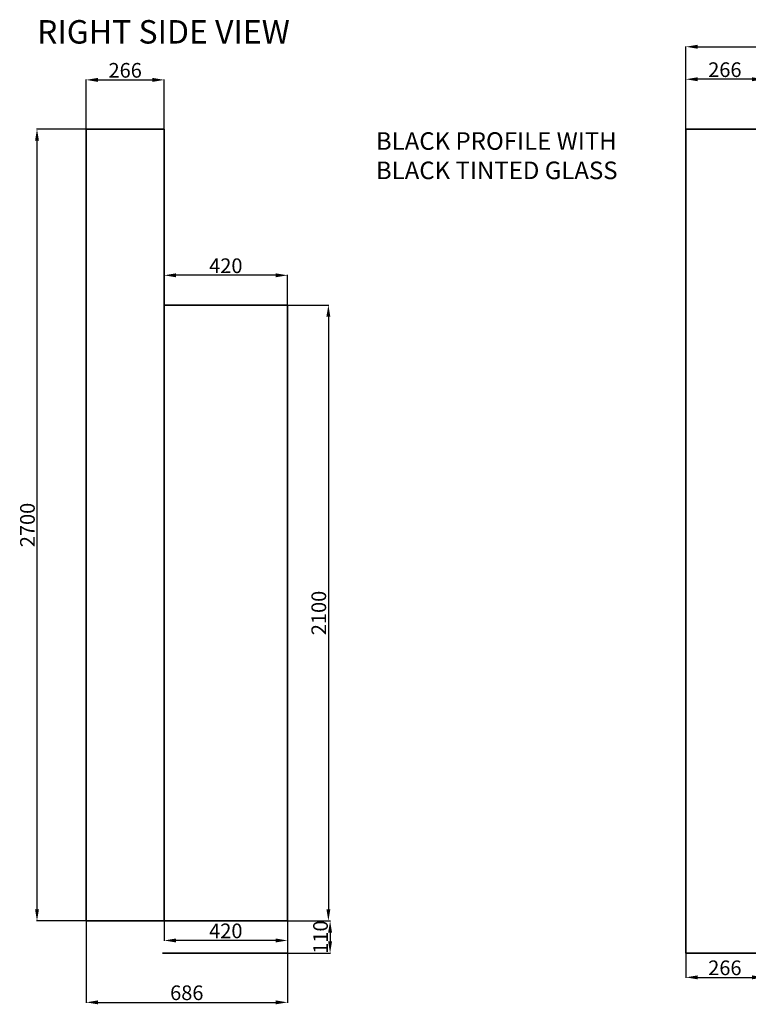
# Model space of a CAD drawing. Units: millimetres. Extents: x 11439 to 24661, y -4767 to -6.
# Tile 1 of 5: x 11439 to 13922, y -4274 to -917. Entities that reach past the tile are written whole.
import ezdxf

# ---------------------------------------------------------------- set-up
doc = ezdxf.new("R2010")
doc.units = ezdxf.units.MM
for name, color, linetype, lineweight in [('A-ANNO-DIMS', 2, 'Continuous', 18), ('A-ANNO-TEXT', 3, 'Continuous', 18), ('A-FURN', 7, 'Continuous', 35)]:
    doc.layers.add(name, color=color, linetype=linetype, lineweight=lineweight)
doc.styles.get("Standard").update_dxf_attribs({"font": 'arial.ttf'})
doc.dimstyles.new('ISO-25', dxfattribs={"dimtxt": 50, "dimasz": 40, "dimexe": 1.25, "dimexo": 0.625, "dimtad": 1, "dimtxsty": 'Standard', "dimcen": 2.5, "dimadec": 0, "dimazin": 0, "dimtfac": 1, "dimtmove": 0, "dimatfit": 3, "dimfxl": 1, "dimarcsym": 0})

# ---------------------------------------------------------------- blocks, each defined once
blk = doc.blocks.new('*D1')
at = {"layer": 'A-ANNO-DIMS', "color": 0, "lineweight": -2, "transparency": 16777216}
for p, q in [((13708.9, -4100.6), (13708.9, -4183.6)), ((13974.9, -4100.6), (13974.9, -4183.6)), ((13748.9, -4182.3), (13934.9, -4182.3))]:
    blk.add_line(p, q, dxfattribs=at)
at = {"layer": 'A-ANNO-DIMS', "color": 0, "transparency": 16777216}
for points in [[(13748.9, -4175.7), (13748.9, -4189), (13708.9, -4182.3)], [(13934.9, -4175.7), (13934.9, -4189), (13974.9, -4182.3)]]:
    blk.add_solid(points, dxfattribs=at)
at = {"layer": 'Defpoints', "color": 0, "transparency": 16777216}
for p in [(13708.9, -4100), (13974.9, -4100), (13974.9, -4182.3)]:
    blk.add_point(p, dxfattribs=at)
at = {"layer": 'A-ANNO-DIMS', "color": 0, "transparency": 16777216, "insert": (13841.9, -4156.2), "char_height": 50, "attachment_point": 5}
blk.add_mtext('266', dxfattribs=at)
blk = doc.blocks.new('*D12')
at = {"layer": 'A-ANNO-DIMS', "color": 0, "lineweight": -2, "transparency": 16777216}
for p, q in [((13708.9, -1289.4), (13708.9, -1119.1)), ((13934.9, -1120.3), (13748.9, -1120.3)), ((13974.9, -1289.4), (13974.9, -1119.1))]:
    blk.add_line(p, q, dxfattribs=at)
at = {"layer": 'A-ANNO-DIMS', "color": 0, "transparency": 16777216}
for points in [[(13748.9, -1113.7), (13748.9, -1127), (13708.9, -1120.3)], [(13934.9, -1113.7), (13934.9, -1127), (13974.9, -1120.3)]]:
    blk.add_solid(points, dxfattribs=at)
at = {"layer": 'Defpoints', "color": 0, "transparency": 16777216}
for p in [(13708.9, -1120.3), (13708.9, -1290), (13974.9, -1290)]:
    blk.add_point(p, dxfattribs=at)
at = {"layer": 'A-ANNO-DIMS', "color": 0, "transparency": 16777216, "insert": (13841.9, -1094.2), "char_height": 50, "attachment_point": 5}
blk.add_mtext('266', dxfattribs=at)
blk = doc.blocks.new('*D17')
at = {"layer": 'A-ANNO-DIMS', "color": 0, "lineweight": -2, "transparency": 16777216}
for p, q in [((12351.7, -1890), (12491.8, -1890)), ((12490.6, -1930), (12490.6, -3950)), ((12351.7, -3990), (12491.8, -3990))]:
    blk.add_line(p, q, dxfattribs=at)
at = {"layer": 'A-ANNO-DIMS', "color": 0, "transparency": 16777216}
for points in [[(12483.9, -1930), (12497.3, -1930), (12490.6, -1890)], [(12483.9, -3950), (12497.3, -3950), (12490.6, -3990)]]:
    blk.add_solid(points, dxfattribs=at)
at = {"layer": 'Defpoints', "color": 0, "transparency": 16777216}
for p in [(12351.1, -1890), (12351.1, -3990), (12490.6, -3990)]:
    blk.add_point(p, dxfattribs=at)
at = {"layer": 'A-ANNO-DIMS', "color": 0, "transparency": 16777216, "insert": (12464.4, -2940), "char_height": 50, "attachment_point": 5, "rotation": 90}
blk.add_mtext('2100', dxfattribs=at)
blk = doc.blocks.new('*D18')
at = {"layer": 'A-ANNO-DIMS', "color": 0, "lineweight": -2, "transparency": 16777216}
for p, q in [((11931.1, -1889.4), (11931.1, -1787.5)), ((12311.1, -1788.7), (11971.1, -1788.7)), ((12351.1, -1889.4), (12351.1, -1787.5))]:
    blk.add_line(p, q, dxfattribs=at)
at = {"layer": 'A-ANNO-DIMS', "color": 0, "transparency": 16777216}
for points in [[(11971.1, -1782), (11971.1, -1795.4), (11931.1, -1788.7)], [(12311.1, -1782), (12311.1, -1795.4), (12351.1, -1788.7)]]:
    blk.add_solid(points, dxfattribs=at)
at = {"layer": 'Defpoints', "color": 0, "transparency": 16777216}
for p in [(11931.1, -1788.7), (11931.1, -1890), (12351.1, -1890)]:
    blk.add_point(p, dxfattribs=at)
at = {"layer": 'A-ANNO-DIMS', "color": 0, "transparency": 16777216, "insert": (12141.1, -1762.6), "char_height": 50, "attachment_point": 5}
blk.add_mtext('420', dxfattribs=at)
blk = doc.blocks.new('*D19')
at = {"layer": 'A-ANNO-DIMS', "color": 0, "lineweight": -2, "transparency": 16777216}
for p, q in [((12351.7, -3990), (12497.7, -3990)), ((12496.5, -4030), (12496.5, -4060)), ((12351.7, -4100), (12497.7, -4100))]:
    blk.add_line(p, q, dxfattribs=at)
at = {"layer": 'A-ANNO-DIMS', "color": 0, "transparency": 16777216}
for points in [[(12489.8, -4030), (12503.1, -4030), (12496.5, -3990)], [(12489.8, -4060), (12503.1, -4060), (12496.5, -4100)]]:
    blk.add_solid(points, dxfattribs=at)
at = {"layer": 'Defpoints', "color": 0, "transparency": 16777216}
for p in [(12351.1, -3990), (12351.1, -4100), (12496.5, -4100)]:
    blk.add_point(p, dxfattribs=at)
at = {"layer": 'A-ANNO-DIMS', "color": 0, "transparency": 16777216, "insert": (12470.3, -4045), "char_height": 50, "attachment_point": 5, "rotation": 90}
blk.add_mtext('110', dxfattribs=at)
blk = doc.blocks.new('*D20')
at = {"layer": 'A-ANNO-DIMS', "color": 0, "lineweight": -2, "transparency": 16777216}
for p, q in [((11931.1, -3990.6), (11931.1, -4057.7)), ((12351.1, -3990.6), (12351.1, -4057.7)), ((12311.1, -4056.5), (11971.1, -4056.5))]:
    blk.add_line(p, q, dxfattribs=at)
at = {"layer": 'A-ANNO-DIMS', "color": 0, "transparency": 16777216}
for points in [[(11971.1, -4049.8), (11971.1, -4063.2), (11931.1, -4056.5)], [(12311.1, -4049.8), (12311.1, -4063.2), (12351.1, -4056.5)]]:
    blk.add_solid(points, dxfattribs=at)
at = {"layer": 'Defpoints', "color": 0, "transparency": 16777216}
for p in [(11931.1, -3990), (12351.1, -3990), (11931.1, -4056.5)]:
    blk.add_point(p, dxfattribs=at)
at = {"layer": 'A-ANNO-DIMS', "color": 0, "transparency": 16777216, "insert": (12141.1, -4030.3), "char_height": 50, "attachment_point": 5}
blk.add_mtext('420', dxfattribs=at)
blk = doc.blocks.new('*D51')
at = {"layer": 'A-ANNO-DIMS', "color": 0, "lineweight": -2, "transparency": 16777216}
for p, q in [((11665.1, -1289.4), (11665.1, -1121.2)), ((11705.1, -1122.5), (11891.1, -1122.5)), ((11931.1, -1289.4), (11931.1, -1121.2))]:
    blk.add_line(p, q, dxfattribs=at)
at = {"layer": 'A-ANNO-DIMS', "color": 0, "transparency": 16777216}
for points in [[(11705.1, -1115.8), (11705.1, -1129.2), (11665.1, -1122.5)], [(11891.1, -1115.8), (11891.1, -1129.2), (11931.1, -1122.5)]]:
    blk.add_solid(points, dxfattribs=at)
at = {"layer": 'Defpoints', "color": 0, "transparency": 16777216}
for p in [(11931.1, -1122.5), (11665.1, -1290), (11931.1, -1290)]:
    blk.add_point(p, dxfattribs=at)
at = {"layer": 'A-ANNO-DIMS', "color": 0, "transparency": 16777216, "insert": (11798.1, -1096.3), "char_height": 50, "attachment_point": 5}
blk.add_mtext('266', dxfattribs=at)
blk = doc.blocks.new('*D52')
at = {"layer": 'A-ANNO-DIMS', "color": 0, "lineweight": -2, "transparency": 16777216}
for p, q in [((11664.5, -1290), (11496.4, -1290)), ((11497.6, -1330), (11497.6, -3950)), ((11664.5, -3990), (11496.4, -3990))]:
    blk.add_line(p, q, dxfattribs=at)
at = {"layer": 'A-ANNO-DIMS', "color": 0, "transparency": 16777216}
for points in [[(11490.9, -1330), (11504.3, -1330), (11497.6, -1290)], [(11490.9, -3950), (11504.3, -3950), (11497.6, -3990)]]:
    blk.add_solid(points, dxfattribs=at)
at = {"layer": 'Defpoints', "color": 0, "transparency": 16777216}
for p in [(11665.1, -1290), (11497.6, -3990), (11665.1, -3990)]:
    blk.add_point(p, dxfattribs=at)
at = {"layer": 'A-ANNO-DIMS', "color": 0, "transparency": 16777216, "insert": (11471.5, -2640), "char_height": 50, "attachment_point": 5, "rotation": 90}
blk.add_mtext('2700', dxfattribs=at)
blk = doc.blocks.new('*D53')
at = {"layer": 'A-ANNO-DIMS', "color": 0, "lineweight": -2, "transparency": 16777216}
for p, q in [((11665.1, -3990.6), (11665.1, -4268.7)), ((12351.1, -3990.6), (12351.1, -4268.7)), ((11705.1, -4267.5), (12311.1, -4267.5))]:
    blk.add_line(p, q, dxfattribs=at)
at = {"layer": 'A-ANNO-DIMS', "color": 0, "transparency": 16777216}
for points in [[(11705.1, -4260.8), (11705.1, -4274.2), (11665.1, -4267.5)], [(12311.1, -4260.8), (12311.1, -4274.2), (12351.1, -4267.5)]]:
    blk.add_solid(points, dxfattribs=at)
at = {"layer": 'Defpoints', "color": 0, "transparency": 16777216}
for p in [(11665.1, -3990), (12351.1, -3990), (12351.1, -4267.5)]:
    blk.add_point(p, dxfattribs=at)
at = {"layer": 'A-ANNO-DIMS', "color": 0, "transparency": 16777216, "insert": (12008.1, -4241.3), "char_height": 50, "attachment_point": 5}
blk.add_mtext('686', dxfattribs=at)
blk = doc.blocks.new('*D58')
at = {"layer": 'A-ANNO-DIMS', "color": 0, "lineweight": -2, "transparency": 16777216}
for p, q in [((13708.9, -1289.4), (13708.9, -1008.2)), ((13748.9, -1009.5), (17164.9, -1009.5)), ((17204.9, -1289.4), (17204.9, -1008.2))]:
    blk.add_line(p, q, dxfattribs=at)
at = {"layer": 'A-ANNO-DIMS', "color": 0, "transparency": 16777216}
for points in [[(13748.9, -1002.8), (13748.9, -1016.2), (13708.9, -1009.5)], [(17164.9, -1002.8), (17164.9, -1016.2), (17204.9, -1009.5)]]:
    blk.add_solid(points, dxfattribs=at)
at = {"layer": 'Defpoints', "color": 0, "transparency": 16777216}
for p in [(17204.9, -1009.5), (13708.9, -1290), (17204.9, -1290)]:
    blk.add_point(p, dxfattribs=at)
at = {"layer": 'A-ANNO-DIMS', "color": 0, "transparency": 16777216, "insert": (15456.9, -983.3), "char_height": 50, "attachment_point": 5}
blk.add_mtext('3496', dxfattribs=at)

msp = doc.modelspace()

# ---------------------------------------------------------------- linework, layer by layer
at = {"layer": 'A-FURN'}
for p, q in [((11931.105, -1289.995), (11665.105, -1289.995)), ((11665.105, -1289.995), (11665.105, -3989.995)), ((11931.105, -1289.995), (11931.105, -3989.995)), ((13708.915, -1289.995), (13708.915, -4099.995)), ((13708.915, -1289.995), (17204.915, -1289.995)), ((12351.105, -1889.995), (11931.105, -1889.995)), ((12351.105, -1889.995), (12351.105, -3989.995)), ((12351.105, -3989.995), (11665.105, -3989.995)), ((12351.105, -4099.995), (11924.983, -4099.995)), ((13708.915, -4099.995), (17204.915, -4099.995)), ((13974.915, -4099.995), (13708.915, -4099.995))]:
    msp.add_line(p, q, dxfattribs=at)

# ---------------------------------------------------------------- texts
at = {"layer": 'A-ANNO-TEXT', "attachment_point": 1}
for s, insert, char_height in [('RIGHT SIDE VIEW', (11497.817, -918.684), 80), (' BLACK PROFILE WITH\\P BLACK TINTED GLASS', (12634.186, -1300.938), 60)]:
    msp.add_mtext_dynamic_manual_height_columns(s, width=1074.7282, gutter_width=12.5, heights=[0], dxfattribs=dict(at, insert=insert, char_height=char_height))

# ---------------------------------------------------------------- dimensions: what is measured, and where the dimension line sits
at = {"layer": 'A-ANNO-DIMS'}
for base, p1, p2, override, picture, middle in [((17204.915, -1009.495), (13708.915, -1289.995), (17204.915, -1289.995), {"dimdec": 0, "dimlfac": 1, "dimrnd": 0, "dimzin": 0, "dimdsep": 46, "dimlunit": 2}, '*D58', (15456.915, -983.325)), ((11931.105, -1122.495), (11665.105, -1289.995), (11931.105, -1289.995), {"dimdec": 0, "dimlfac": 1, "dimrnd": 0, "dimzin": 0, "dimdsep": 46, "dimlunit": 2}, '*D51', (11798.105, -1096.342)), ((13708.915, -1120.332), (13974.915, -1289.995), (13708.915, -1289.995), {"dimclrd": 0, "dimclre": 0, "dimclrt": 0}, '*D12', (13841.915, -1094.178)), ((11931.105, -1788.709), (12351.105, -1889.995), (11931.105, -1889.995), {"dimclrd": 0, "dimclre": 0, "dimclrt": 0}, '*D18', (12141.105, -1762.556)), ((12351.105, -4267.495), (11665.105, -3989.995), (12351.105, -3989.995), {"dimdec": 0, "dimlfac": 1, "dimrnd": 0, "dimzin": 0, "dimdsep": 46, "dimlunit": 2}, '*D53', (12008.105, -4241.342)), ((11931.105, -4056.49), (12351.105, -3989.995), (11931.105, -3989.995), {"dimclrd": 0, "dimclre": 0, "dimclrt": 0}, '*D20', (12141.105, -4030.337)), ((13974.915, -4182.342), (13708.915, -4099.995), (13974.915, -4099.995), {"dimclrd": 0, "dimclre": 0, "dimclrt": 0}, '*D1', (13841.915, -4156.188))]:
    dim = msp.add_linear_dim(base=base, p1=p1, p2=p2, dimstyle='ISO-25', override=override, dxfattribs=at)
    dim.commit()
    dim.dimension.update_dxf_attribs({"geometry": picture, "text_midpoint": middle})
for base, p1, p2, override, picture, middle in [((11497.605, -3989.995), (11665.105, -1289.995), (11665.105, -3989.995), {"dimdec": 0, "dimlfac": 1, "dimrnd": 0, "dimzin": 0, "dimdsep": 46, "dimlunit": 2}, '*D52', (11471.452, -2639.995)), ((12490.589, -3989.995), (12351.105, -1889.995), (12351.105, -3989.995), {"dimclrd": 0, "dimclre": 0, "dimclrt": 0}, '*D17', (12464.436, -2939.995)), ((12496.472, -4099.995), (12351.105, -3989.995), (12351.105, -4099.995), {"dimclrd": 0, "dimclre": 0, "dimclrt": 0}, '*D19', (12470.318, -4044.995))]:
    dim = msp.add_linear_dim(base=base, p1=p1, p2=p2, angle=90, dimstyle='ISO-25', override=override, dxfattribs=at)
    dim.commit()
    dim.dimension.update_dxf_attribs({"geometry": picture, "text_midpoint": middle})

doc.saveas('drawing.dxf')
